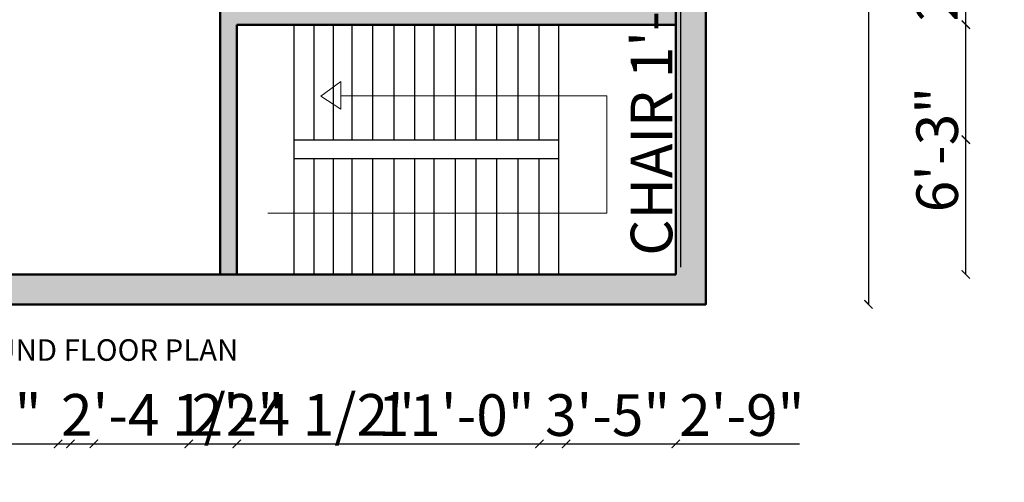
# Model space of a CAD drawing. Units: inches. Extents: x 2419 to 2878, y 1068 to 1713.
# Tile 8 of 20: x 2574 to 2870, y 1068 to 1207. Entities that reach past the tile are written whole.
import ezdxf

# ---------------------------------------------------------------- set-up
doc = ezdxf.new("R2010")
doc.units = ezdxf.units.IN
for name, color, linetype, lineweight in [('A-ANNO-DIMS', 2, 'Continuous', 18), ('A-ANNO-SYMB', 3, 'Continuous', 18), ('A-ANNO-TEXT', 7, 'Continuous', 25), ('A-FLOR-PRKG-PATT', 1, 'Continuous', 13), ('A-FLOR-STRS', 7, 'Continuous', 25), ('A-WALL', 7, 'Continuous', 50)]:
    doc.layers.add(name, color=color, linetype=linetype, lineweight=lineweight)
doc.layers.add('A-WALL-PATT', color=18, linetype='Continuous', lineweight=13, true_color=0x000000)
doc.styles.get("Standard").update_dxf_attribs({"font": 'arial.ttf'})
doc.dimstyles.new('ISO-25', dxfattribs={"dimtxt": 12.5, "dimasz": 2.5, "dimexe": 1.25, "dimexo": 0.625, "dimtad": 1, "dimdec": 0, "dimlunit": 4, "dimtxsty": 'Standard', "dimblk": 'ARCHTICK', "dimcen": 2.5, "dimse1": 1, "dimse2": 1, "dimclrd": 4, "dimadec": 0, "dimazin": 0, "dimtfac": 1, "dimtdec": 0, "dimtmove": 0, "dimatfit": 3, "dimfxl": 1, "dimarcsym": 0})

# ---------------------------------------------------------------- blocks, each defined once
blk = doc.blocks.new('_ArchTick')
at = {"color": 0, "linetype": 'ByBlock', "const_width": 0.15}
blk.add_lwpolyline([(-0.5, -0.5), (0.5, 0.5)], dxfattribs=at)
blk = doc.blocks.new('*D17')
at = {"layer": 'A-ANNO-DIMS', "color": 0, "lineweight": -2, "transparency": 16777216}
blk.add_line((2829.44, 1577.81), (2829.44, 1121.81), dxfattribs=at)
at = {"layer": 'Defpoints', "color": 0, "transparency": 16777216}
for p in [(2780.51, 1577.81), (2780.51, 1121.81), (2829.44, 1121.81)]:
    blk.add_point(p, dxfattribs=at)
at = {"layer": 'A-ANNO-DIMS', "color": 0, "lineweight": -2, "transparency": 16777216, "xscale": 2.5, "yscale": 2.5, "zscale": 2.5}
for p, rotation in [((2829.44, 1577.81), 90), ((2829.44, 1121.81), 270)]:
    blk.add_blockref('_ArchTick', p, dxfattribs=dict(at, rotation=rotation))
at = {"layer": 'A-ANNO-DIMS', "color": 0, "transparency": 16777216, "insert": (2822.42, 1349.81), "char_height": 12.5, "attachment_point": 5, "rotation": 90}
blk.add_mtext("38'", dxfattribs=at)
blk = doc.blocks.new('*D18')
at = {"layer": 'A-ANNO-DIMS', "color": 4, "lineweight": -2, "transparency": 16777216}
for p, q in [((2772.91, 1292.99), (2772.91, 1271.99)), ((2772.91, 1271.99), (2772.91, 1133))]:
    blk.add_line(p, q, dxfattribs=at)
at = {"layer": 'Defpoints', "color": 0, "transparency": 16777216}
for p in [(2769.76, 1292.99), (2769.76, 1271.99), (2772.91, 1271.99)]:
    blk.add_point(p, dxfattribs=at)
at = {"layer": 'A-ANNO-DIMS', "color": 4, "lineweight": -2, "transparency": 16777216, "xscale": 2.5, "yscale": 2.5, "zscale": 2.5}
for p, rotation in [((2772.91, 1292.99), 90), ((2772.91, 1271.99), 270)]:
    blk.add_blockref('_ArchTick', p, dxfattribs=dict(at, rotation=rotation))
at = {"layer": 'A-ANNO-DIMS', "color": 0, "transparency": 16777216, "insert": (2765.82, 1201.24), "char_height": 12.5, "attachment_point": 5, "rotation": 90}
blk.add_mtext('CHAIR 1\'-9" TYP.', dxfattribs=at)
blk = doc.blocks.new('*D34')
at = {"layer": 'A-ANNO-DIMS', "color": 4, "lineweight": -2, "transparency": 16777216}
blk.add_line((2639.51, 1079.92), (2771.51, 1079.92), dxfattribs=at)
at = {"layer": 'Defpoints', "color": 0, "transparency": 16777216}
for p in [(2639.51, 1130.81), (2771.51, 1130.81), (2771.51, 1079.92)]:
    blk.add_point(p, dxfattribs=at)
at = {"layer": 'A-ANNO-DIMS', "color": 4, "lineweight": -2, "transparency": 16777216, "xscale": 2.5, "yscale": 2.5, "zscale": 2.5, "rotation": 180}
blk.add_blockref('_ArchTick', (2639.51, 1079.92), dxfattribs=at)
at = {"layer": 'A-ANNO-DIMS', "color": 4, "lineweight": -2, "transparency": 16777216, "xscale": 2.5, "yscale": 2.5, "zscale": 2.5}
blk.add_blockref('_ArchTick', (2771.51, 1079.92), dxfattribs=at)
at = {"layer": 'A-ANNO-DIMS', "color": 0, "transparency": 16777216, "insert": (2705.51, 1086.93), "char_height": 12.5, "attachment_point": 5}
blk.add_mtext('11\'-0"', dxfattribs=at)
blk = doc.blocks.new('*D35')
at = {"layer": 'A-ANNO-DIMS', "color": 4, "lineweight": -2, "transparency": 16777216}
blk.add_line((2858.71, 1130.81), (2858.71, 1205.81), dxfattribs=at)
at = {"layer": 'Defpoints', "color": 0, "transparency": 16777216}
for p in [(2771.51, 1205.81), (2858.71, 1205.81), (2771.51, 1130.81)]:
    blk.add_point(p, dxfattribs=at)
at = {"layer": 'A-ANNO-DIMS', "color": 4, "lineweight": -2, "transparency": 16777216, "xscale": 2.5, "yscale": 2.5, "zscale": 2.5}
for p, rotation in [((2858.71, 1205.81), 90), ((2858.71, 1130.81), 270)]:
    blk.add_blockref('_ArchTick', p, dxfattribs=dict(at, rotation=rotation))
at = {"layer": 'A-ANNO-DIMS', "color": 0, "transparency": 16777216, "insert": (2851.7, 1168.31), "char_height": 12.5, "attachment_point": 5, "rotation": 90}
blk.add_mtext('6\'-3"', dxfattribs=at)
blk = doc.blocks.new('*D36')
at = {"layer": 'A-ANNO-DIMS', "color": 4, "lineweight": -2, "transparency": 16777216}
blk.add_line((2656.74, 1605.01), (2736.32, 1605.01), dxfattribs=at)
at = {"layer": 'Defpoints', "color": 0, "transparency": 16777216}
for p in [(2736.32, 1605.01), (2656.74, 1205.81), (2736.32, 1205.81)]:
    blk.add_point(p, dxfattribs=at)
at = {"layer": 'A-ANNO-DIMS', "color": 4, "lineweight": -2, "transparency": 16777216, "xscale": 2.5, "yscale": 2.5, "zscale": 2.5, "rotation": 180}
blk.add_blockref('_ArchTick', (2656.74, 1605.01), dxfattribs=at)
at = {"layer": 'A-ANNO-DIMS', "color": 4, "lineweight": -2, "transparency": 16777216, "xscale": 2.5, "yscale": 2.5, "zscale": 2.5}
blk.add_blockref('_ArchTick', (2736.32, 1605.01), dxfattribs=at)
at = {"layer": 'A-ANNO-DIMS', "color": 0, "transparency": 16777216, "insert": (2696.53, 1612.1), "char_height": 12.5, "attachment_point": 5}
blk.add_mtext('6\'-7 1/2"', dxfattribs=at)
blk = doc.blocks.new('*D37')
at = {"layer": 'A-ANNO-DIMS', "color": 4, "lineweight": -2, "transparency": 16777216}
for p, q in [((2736.32, 1605.01), (2771.51, 1605.01)), ((2771.51, 1605.01), (2818.42, 1605.01))]:
    blk.add_line(p, q, dxfattribs=at)
at = {"layer": 'Defpoints', "color": 0, "transparency": 16777216}
for p in [(2771.51, 1605.01), (2736.32, 1205.81), (2771.51, 1205.81)]:
    blk.add_point(p, dxfattribs=at)
at = {"layer": 'A-ANNO-DIMS', "color": 4, "lineweight": -2, "transparency": 16777216, "xscale": 2.5, "yscale": 2.5, "zscale": 2.5, "rotation": 180}
blk.add_blockref('_ArchTick', (2736.32, 1605.01), dxfattribs=at)
at = {"layer": 'A-ANNO-DIMS', "color": 4, "lineweight": -2, "transparency": 16777216, "xscale": 2.5, "yscale": 2.5, "zscale": 2.5}
blk.add_blockref('_ArchTick', (2771.51, 1605.01), dxfattribs=at)
at = {"layer": 'A-ANNO-DIMS', "color": 0, "transparency": 16777216, "insert": (2796.22, 1611.91), "char_height": 12.5, "attachment_point": 5}
blk.add_mtext('2\'-11"', dxfattribs=at)
blk = doc.blocks.new('*D38')
at = {"layer": 'A-ANNO-DIMS', "color": 4, "lineweight": -2, "transparency": 16777216}
for p, q in [((2444.31, 1165.6), (2444.31, 1212.51)), ((2444.31, 1130.81), (2444.31, 1165.6))]:
    blk.add_line(p, q, dxfattribs=at)
at = {"layer": 'Defpoints', "color": 0, "transparency": 16777216}
for p in [(2444.31, 1165.6), (2656.74, 1165.6), (2656.74, 1130.81)]:
    blk.add_point(p, dxfattribs=at)
at = {"layer": 'A-ANNO-DIMS', "color": 4, "lineweight": -2, "transparency": 16777216, "xscale": 2.5, "yscale": 2.5, "zscale": 2.5}
for p, rotation in [((2444.31, 1165.6), 90), ((2444.31, 1130.81), 270)]:
    blk.add_blockref('_ArchTick', p, dxfattribs=dict(at, rotation=rotation))
at = {"layer": 'A-ANNO-DIMS', "color": 0, "transparency": 16777216, "insert": (2437.41, 1190.3), "char_height": 12.5, "attachment_point": 5, "rotation": 90}
blk.add_mtext('2\'-11"', dxfattribs=at)
blk = doc.blocks.new('*D39')
at = {"layer": 'A-ANNO-DIMS', "color": 4, "lineweight": -2, "transparency": 16777216}
for p, q in [((2662.74, 1605.01), (2668.59, 1605.01)), ((2668.59, 1605.01), (2705.56, 1605.01))]:
    blk.add_line(p, q, dxfattribs=at)
at = {"layer": 'Defpoints', "color": 0, "transparency": 16777216}
for p in [(2668.59, 1605.01), (2662.74, 1165.6), (2668.59, 1165.6)]:
    blk.add_point(p, dxfattribs=at)
at = {"layer": 'A-ANNO-DIMS', "color": 4, "lineweight": -2, "transparency": 16777216, "xscale": 2.5, "yscale": 2.5, "zscale": 2.5, "rotation": 180}
blk.add_blockref('_ArchTick', (2662.74, 1605.01), dxfattribs=at)
at = {"layer": 'A-ANNO-DIMS', "color": 4, "lineweight": -2, "transparency": 16777216, "xscale": 2.5, "yscale": 2.5, "zscale": 2.5}
blk.add_blockref('_ArchTick', (2668.59, 1605.01), dxfattribs=at)
at = {"layer": 'A-ANNO-DIMS', "color": 0, "transparency": 16777216, "insert": (2688.32, 1612.02), "char_height": 12.5, "attachment_point": 5}
blk.add_mtext('0\'-6"', dxfattribs=at)
blk = doc.blocks.new('*D40')
at = {"layer": 'A-ANNO-DIMS', "color": 4, "lineweight": -2, "transparency": 16777216}
for p, q in [((2858.71, 1205.81), (2858.71, 1281.84)), ((2858.71, 1171.28), (2858.71, 1205.81))]:
    blk.add_line(p, q, dxfattribs=at)
at = {"layer": 'Defpoints', "color": 0, "transparency": 16777216}
for p in [(2736.32, 1205.81), (2858.71, 1205.81), (2736.32, 1171.28)]:
    blk.add_point(p, dxfattribs=at)
at = {"layer": 'A-ANNO-DIMS', "color": 4, "lineweight": -2, "transparency": 16777216, "xscale": 2.5, "yscale": 2.5, "zscale": 2.5}
for p, rotation in [((2858.71, 1205.81), 90), ((2858.71, 1171.28), 270)]:
    blk.add_blockref('_ArchTick', p, dxfattribs=dict(at, rotation=rotation))
at = {"layer": 'A-ANNO-DIMS', "color": 0, "transparency": 16777216, "insert": (2851.63, 1245.08), "char_height": 12.5, "attachment_point": 5, "rotation": 90}
blk.add_mtext('2\'-10 1/2"', dxfattribs=at)
blk = doc.blocks.new('*D44')
at = {"layer": 'A-ANNO-DIMS', "color": 4, "lineweight": -2, "transparency": 16777216}
for p, q in [((2557.3, 1079.92), (2585.82, 1079.92)), ((2585.82, 1079.92), (2652.14, 1079.92))]:
    blk.add_line(p, q, dxfattribs=at)
at = {"layer": 'Defpoints', "color": 0, "transparency": 16777216}
for p in [(2557.3, 1408.81), (2585.82, 1408.81), (2585.82, 1079.92)]:
    blk.add_point(p, dxfattribs=at)
at = {"layer": 'A-ANNO-DIMS', "color": 4, "lineweight": -2, "transparency": 16777216, "xscale": 2.5, "yscale": 2.5, "zscale": 2.5, "rotation": 180}
blk.add_blockref('_ArchTick', (2557.3, 1079.92), dxfattribs=at)
at = {"layer": 'A-ANNO-DIMS', "color": 4, "lineweight": -2, "transparency": 16777216, "xscale": 2.5, "yscale": 2.5, "zscale": 2.5}
blk.add_blockref('_ArchTick', (2585.82, 1079.92), dxfattribs=at)
at = {"layer": 'A-ANNO-DIMS', "color": 0, "transparency": 16777216, "insert": (2620.23, 1087.01), "char_height": 12.5, "attachment_point": 5}
blk.add_mtext('2\'-4 1/2"', dxfattribs=at)
blk = doc.blocks.new('*D45')
at = {"layer": 'A-ANNO-DIMS', "color": 4, "lineweight": -2, "transparency": 16777216}
for p, q in [((2596.57, 1079.92), (2625.09, 1079.92)), ((2625.09, 1079.92), (2691.41, 1079.92))]:
    blk.add_line(p, q, dxfattribs=at)
at = {"layer": 'Defpoints', "color": 0, "transparency": 16777216}
for p in [(2596.57, 1408.81), (2625.09, 1408.81), (2625.09, 1079.92)]:
    blk.add_point(p, dxfattribs=at)
at = {"layer": 'A-ANNO-DIMS', "color": 4, "lineweight": -2, "transparency": 16777216, "xscale": 2.5, "yscale": 2.5, "zscale": 2.5, "rotation": 180}
blk.add_blockref('_ArchTick', (2596.57, 1079.92), dxfattribs=at)
at = {"layer": 'A-ANNO-DIMS', "color": 4, "lineweight": -2, "transparency": 16777216, "xscale": 2.5, "yscale": 2.5, "zscale": 2.5}
blk.add_blockref('_ArchTick', (2625.09, 1079.92), dxfattribs=at)
at = {"layer": 'A-ANNO-DIMS', "color": 0, "transparency": 16777216, "insert": (2659.5, 1087.01), "char_height": 12.5, "attachment_point": 5}
blk.add_mtext('2\'-4 1/2"', dxfattribs=at)
blk = doc.blocks.new('*D51')
at = {"layer": 'A-ANNO-DIMS', "color": 4, "lineweight": -2, "transparency": 16777216}
for p, q in [((2738.51, 1079.92), (2771.51, 1079.92)), ((2771.51, 1079.92), (2808.71, 1079.92))]:
    blk.add_line(p, q, dxfattribs=at)
at = {"layer": 'Defpoints', "color": 0, "transparency": 16777216}
for p in [(2738.51, 1447.89), (2771.51, 1437.39), (2771.51, 1079.92)]:
    blk.add_point(p, dxfattribs=at)
at = {"layer": 'A-ANNO-DIMS', "color": 4, "lineweight": -2, "transparency": 16777216, "xscale": 2.5, "yscale": 2.5, "zscale": 2.5, "rotation": 180}
blk.add_blockref('_ArchTick', (2738.51, 1079.92), dxfattribs=at)
at = {"layer": 'A-ANNO-DIMS', "color": 4, "lineweight": -2, "transparency": 16777216, "xscale": 2.5, "yscale": 2.5, "zscale": 2.5}
blk.add_blockref('_ArchTick', (2771.51, 1079.92), dxfattribs=at)
at = {"layer": 'A-ANNO-DIMS', "color": 0, "transparency": 16777216, "insert": (2791.36, 1086.93), "char_height": 12.5, "attachment_point": 5}
blk.add_mtext('2\'-9"', dxfattribs=at)
blk = doc.blocks.new('*D56')
at = {"layer": 'A-ANNO-DIMS', "color": 4, "lineweight": -2, "transparency": 16777216}
for p, q in [((2480.51, 1079.92), (2503.97, 1079.92)), ((2503.97, 1079.92), (2578.61, 1079.92))]:
    blk.add_line(p, q, dxfattribs=at)
at = {"layer": 'Defpoints', "color": 0, "transparency": 16777216}
for p in [(2480.51, 1507.81), (2503.97, 1494.85), (2503.97, 1079.92)]:
    blk.add_point(p, dxfattribs=at)
at = {"layer": 'A-ANNO-DIMS', "color": 4, "lineweight": -2, "transparency": 16777216, "xscale": 2.5, "yscale": 2.5, "zscale": 2.5, "rotation": 180}
blk.add_blockref('_ArchTick', (2480.51, 1079.92), dxfattribs=at)
at = {"layer": 'A-ANNO-DIMS', "color": 4, "lineweight": -2, "transparency": 16777216, "xscale": 2.5, "yscale": 2.5, "zscale": 2.5}
blk.add_blockref('_ArchTick', (2503.97, 1079.92), dxfattribs=at)
at = {"layer": 'A-ANNO-DIMS', "color": 0, "transparency": 16777216, "insert": (2542.54, 1087.01), "char_height": 12.5, "attachment_point": 5}
blk.add_mtext('1\'-11 1/2"', dxfattribs=at)
blk = doc.blocks.new('*D59')
at = {"layer": 'A-ANNO-DIMS', "color": 4, "lineweight": -2, "transparency": 16777216}
blk.add_line((2480.51, 1079.92), (2589.51, 1079.92), dxfattribs=at)
at = {"layer": 'Defpoints', "color": 0, "transparency": 16777216}
for p in [(2480.51, 1414.81), (2589.51, 1414.81), (2589.51, 1079.92)]:
    blk.add_point(p, dxfattribs=at)
at = {"layer": 'A-ANNO-DIMS', "color": 4, "lineweight": -2, "transparency": 16777216, "xscale": 2.5, "yscale": 2.5, "zscale": 2.5, "rotation": 180}
blk.add_blockref('_ArchTick', (2480.51, 1079.92), dxfattribs=at)
at = {"layer": 'A-ANNO-DIMS', "color": 4, "lineweight": -2, "transparency": 16777216, "xscale": 2.5, "yscale": 2.5, "zscale": 2.5}
blk.add_blockref('_ArchTick', (2589.51, 1079.92), dxfattribs=at)
at = {"layer": 'A-ANNO-DIMS', "color": 0, "transparency": 16777216, "insert": (2535.01, 1086.93), "char_height": 12.5, "attachment_point": 5}
blk.add_mtext('9\'-1"', dxfattribs=at)
blk = doc.blocks.new('*D61')
at = {"layer": 'A-ANNO-DIMS', "color": 4, "lineweight": -2, "transparency": 16777216}
blk.add_line((2730.51, 1079.92), (2771.51, 1079.92), dxfattribs=at)
at = {"layer": 'Defpoints', "color": 0, "transparency": 16777216}
for p in [(2730.51, 1414.81), (2771.51, 1414.81), (2771.51, 1079.92)]:
    blk.add_point(p, dxfattribs=at)
at = {"layer": 'A-ANNO-DIMS', "color": 4, "lineweight": -2, "transparency": 16777216, "xscale": 2.5, "yscale": 2.5, "zscale": 2.5, "rotation": 180}
blk.add_blockref('_ArchTick', (2730.51, 1079.92), dxfattribs=at)
at = {"layer": 'A-ANNO-DIMS', "color": 4, "lineweight": -2, "transparency": 16777216, "xscale": 2.5, "yscale": 2.5, "zscale": 2.5}
blk.add_blockref('_ArchTick', (2771.51, 1079.92), dxfattribs=at)
at = {"layer": 'A-ANNO-DIMS', "color": 0, "transparency": 16777216, "insert": (2751.01, 1086.94), "char_height": 12.5, "attachment_point": 5}
blk.add_mtext('3\'-5"', dxfattribs=at)

msp = doc.modelspace()

# ---------------------------------------------------------------- hatches: boundary and pattern name
at = {"layer": 'A-FLOR-PRKG-PATT'}
h = msp.add_hatch(color=256, dxfattribs=at)
h.dxf.hatch_style = 1
edge = h.paths.add_edge_path()
edge.add_ellipse((2561.37, 1279.45), major_axis=(3.99, 0), ratio=0.842304, start_angle=0.6466, end_angle=90)
edge.add_line((2561.37, 1282.81), (2511.57, 1282.81))
edge.add_ellipse((2511.57, 1279.45), major_axis=(3.99, 0), ratio=0.842304, start_angle=90, end_angle=179.3534)
edge.add_ellipse((10560.89, 1188.62), major_axis=(-8054.03, 0), ratio=0.8423039, start_angle=-0.646554, end_angle=-0.628237)
edge.add_ellipse((2509.23, 1276.91), major_axis=(1.69, 0), ratio=0.842304, start_angle=179.3718, end_angle=248.4648)
edge.add_ellipse((10560.33, 1188.62), major_axis=(8052.29, 0), ratio=0.8423039, start_angle=179.353446, end_angle=179.381357, ccw=False)
edge.add_ellipse((2511.01, 1279.45), major_axis=(2.25, 0), ratio=0.842304, start_angle=90, end_angle=179.3534, ccw=False)
edge.add_line((2511.01, 1281.35), (2561.94, 1281.35))
edge.add_ellipse((2561.94, 1279.45), major_axis=(-2.25, 0), ratio=0.842304, start_angle=180.6466, end_angle=270, ccw=False)
edge.add_ellipse((-5487.38, 1188.62), major_axis=(8052.29, 0), ratio=0.8423039, start_angle=0.528271, end_angle=0.646554, ccw=False)
edge.add_ellipse((2563.71, 1276.91), major_axis=(-1.69, 0), ratio=0.842304, start_angle=111.5352, end_angle=180.6282)
edge.add_ellipse((-5487.95, 1188.62), major_axis=(-8054.03, 0), ratio=0.8423039, start_angle=180.628237, end_angle=180.646554)
edge = h.paths.add_edge_path()
edge.add_ellipse((2564.91, 1261.91), major_axis=(-1.12, 0), ratio=0.842304, start_angle=180, end_angle=270)
edge.add_line((2564.91, 1262.86), (2564.43, 1262.86))
edge.add_ellipse((-5487.38, 1188.62), major_axis=(8052.29, 0), ratio=0.8423039, start_angle=0.383867, end_angle=0.528271, ccw=False)
edge.add_line((2564.65, 1242.56), (2564.91, 1242.56))
edge.add_ellipse((2564.91, 1243.51), major_axis=(-1.12, 0), ratio=0.842304, start_angle=90, end_angle=180)
edge.add_line((2566.03, 1243.51), (2566.03, 1261.91))
edge = h.paths.add_edge_path()
edge.add_ellipse((2564.91, 1174.99), major_axis=(1.12, 0), ratio=0.842304, start_angle=0, end_angle=90)
edge.add_line((2564.91, 1175.94), (2564.89, 1175.94))
edge.add_ellipse((-5487.38, 1188.62), major_axis=(8052.29, 0), ratio=0.8423039, start_angle=-0.134987, end_angle=-0.090229, ccw=False)
edge.add_ellipse((2163.34, 1170.91), major_axis=(401.54, 0), ratio=0.842304, start_angle=-2.18, end_angle=-0.1356, ccw=False)
edge.add_line((2564.47, 1155.64), (2564.91, 1155.64))
edge.add_ellipse((2564.91, 1156.59), major_axis=(-1.12, 0), ratio=0.842304, start_angle=90, end_angle=180)
edge.add_line((2566.03, 1156.59), (2566.03, 1174.99))
h.paths.add_polyline_path([(2574.48, 1207.45), (2633.94, 1207.45), (2633.94, 1217.37), (2574.48, 1217.37)], flags=9)
h.paths.add_polyline_path([(2574.45, 1217.83), (2610.47, 1217.83), (2610.47, 1227.88), (2574.45, 1227.88)], flags=9)
h.paths.add_polyline_path([(2672.43, 1304.02), (2718.62, 1304.02), (2718.62, 1313.94), (2672.43, 1313.94)], flags=9)
h.paths.add_polyline_path([(2672.4, 1314.4), (2750.13, 1314.4), (2750.13, 1324.45), (2672.4, 1324.45)], flags=9)
h.paths.add_polyline_path([(2500.43, 1374.44), (2544.8, 1374.44), (2544.8, 1384.36), (2500.43, 1384.36)], flags=9)
h.paths.add_polyline_path([(2500.41, 1384.82), (2566.08, 1384.82), (2566.08, 1394.87), (2500.41, 1394.87)], flags=9)
h.paths.add_polyline_path([(2738.93, 1376.75), (2778.27, 1376.75), (2778.27, 1386.67), (2738.93, 1386.67)], flags=9)
h.paths.add_polyline_path([(2659.12, 1357.8), (2703.49, 1357.8), (2703.49, 1367.72), (2659.12, 1367.72)], flags=9)
h.paths.add_polyline_path([(2659.1, 1368.18), (2694.11, 1368.18), (2694.11, 1378.23), (2659.1, 1378.23)], flags=9)
h.paths.add_polyline_path([(2730.12, 1466.07), (2769.46, 1466.07), (2769.46, 1475.99), (2730.12, 1475.99)], flags=9)
h.paths.add_polyline_path([(2730.1, 1476.45), (2765.12, 1476.45), (2765.12, 1486.5), (2730.1, 1486.5)], flags=9)
h.paths.add_polyline_path([(2730.38, 1518.65), (2761.48, 1518.65), (2761.48, 1528.57), (2730.38, 1528.57)], flags=9)
h.paths.add_polyline_path([(2730.36, 1529.03), (2780.96, 1529.03), (2780.96, 1539.07), (2730.36, 1539.07)], flags=9)
h.paths.add_polyline_path([(2629.32, 1455.19), (2688.78, 1455.19), (2688.78, 1465.11), (2629.32, 1465.11)], flags=9)
h.paths.add_polyline_path([(2629.3, 1465.57), (2681.9, 1465.57), (2681.9, 1475.62), (2629.3, 1475.62)], flags=9)
h.paths.add_polyline_path([(2513.23, 1456.48), (2562.63, 1456.48), (2562.63, 1466.4), (2513.23, 1466.4)], flags=9)
h.paths.add_polyline_path([(2513.21, 1466.86), (2556.26, 1466.86), (2556.26, 1476.91), (2513.21, 1476.91)], flags=9)
h.paths.add_polyline_path([(2488.87, 1521.54), (2519.97, 1521.54), (2519.97, 1531.46), (2488.87, 1531.46)], flags=9)
h.paths.add_polyline_path([(2536.55, 1543.51), (2580.92, 1543.51), (2580.92, 1553.43), (2536.55, 1553.43)], flags=9)
h.paths.add_polyline_path([(2536.56, 1553.92), (2573.53, 1553.92), (2573.53, 1563.8), (2536.56, 1563.8)], flags=9)
at = {"layer": 'A-WALL-PATT'}
h = msp.add_hatch(color=256, dxfattribs=at)
h.dxf.hatch_style = 1
h.paths.add_polyline_path([(2780.51, 1577.81), (2471.51, 1577.81), (2471.51, 1121.81), (2780.51, 1121.81)])
h.paths.add_polyline_path([(2480.51, 1568.81), (2771.51, 1568.81), (2771.51, 1130.81), (2480.51, 1130.81)], flags=16)
h.paths.add_polyline_path([(2528.51, 1568.81), (2528.51, 1512.81), (2594.51, 1512.81), (2594.51, 1414.81), (2596.57, 1414.81), (2596.57, 1441.61), (2597.82, 1441.61), (2597.82, 1441.58, -0.384016), (2625.03, 1414.81), (2725.51, 1414.81), (2725.51, 1567.55), (2728.3, 1567.55), (2746.89, 1567.55), (2746.89, 1566.73), (2746.87, 1566.73, -0.367216), (2730.51, 1549.09), (2730.51, 1512.81), (2750.85, 1512.81), (2750.85, 1510.03, -0.401453), (2733.08, 1491.46), (2733.08, 1491.44), (2732.27, 1491.44), (2732.27, 1507.81), (2730.51, 1507.81), (2730.51, 1408.81), (2736.51, 1408.81), (2736.51, 1349.81), (2632.51, 1349.81), (2632.51, 1408.81), (2528.51, 1408.81), (2528.51, 1414.81), (2503.97, 1414.81), (2503.97, 1494.85), (2558.38, 1494.85), (2558.38, 1507.81), (2529.96, 1507.81, -0.414214), (2530.82, 1506.96), (2530.82, 1497.26, -0.414214), (2529.96, 1496.4), (2514.56, 1496.4, -0.414214), (2513.7, 1497.26), (2513.7, 1506.96, -0.414214), (2514.56, 1507.81), (2528.51, 1507.81), (2528.51, 1512.81), (2480.51, 1512.81)], flags=0)
h.paths.add_polyline_path([(2516.26, 1507.81), (2528.26, 1507.81), (2528.26, 1505.81), (2523.42, 1505.81), (2524.07, 1504.67), (2529.39, 1504.67, -0.414214), (2529.96, 1504.1), (2529.96, 1497.83, -0.414214), (2529.39, 1497.26), (2515.13, 1497.26, -0.414214), (2514.56, 1497.83), (2514.56, 1504.1, -0.414214), (2515.13, 1504.67), (2520.69, 1504.67), (2521.34, 1505.81), (2516.26, 1505.81)], flags=0)
h.paths.add_polyline_path([(2522.02, 1505.53), (2522.82, 1507.32, -0.65506), (2522.25, 1506.06), (2522.19, 1505.93), (2522.43, 1505.53)], flags=0)
h.paths.add_polyline_path([(2522.83, 1500.97, -1), (2521.69, 1500.97, -1)], flags=0)
h.paths.add_polyline_path([(2522.55, 1500.97, -1), (2521.98, 1500.97, -1)], flags=0)
h.paths.add_polyline_path([(2482.01, 1470.63), (2499.89, 1470.63), (2499.89, 1448.27), (2482.01, 1448.27), (2482.01, 1452.74), (2481.26, 1452.74), (2481.26, 1449.76), (2480.51, 1449.76), (2480.51, 1469.14), (2481.26, 1469.14), (2481.26, 1466.16), (2482.01, 1466.16)], flags=0)
h.paths.add_polyline_path([(2488.71, 1466.16, -1), (2484.24, 1466.16, -1)], flags=0)
h.paths.add_polyline_path([(2496.17, 1466.16, -1), (2490.2, 1466.16, -1)], flags=0)
h.paths.add_polyline_path([(2487.97, 1466.16, -1), (2484.99, 1466.16, -1)], flags=0)
h.paths.add_polyline_path([(2495.42, 1466.16, -1), (2490.95, 1466.16, -1)], flags=0)
h.paths.add_polyline_path([(2487.22, 1466.16, -1), (2485.73, 1466.16, -1)], flags=0)
h.paths.add_polyline_path([(2494.68, 1466.16, -1), (2491.69, 1466.16, -1)], flags=0)
h.paths.add_polyline_path([(2499.11, 1468, -1), (2497.98, 1468, -1)], flags=0)
h.paths.add_polyline_path([(2493.93, 1466.16, -1), (2492.44, 1466.16, -1)], flags=0)
h.paths.add_polyline_path([(2499.37, 1463.71, -1), (2498.17, 1463.71, -1)], flags=0)
h.paths.add_polyline_path([(2484.24, 1461.69), (2496.17, 1461.69), (2496.17, 1457.22), (2484.24, 1457.22)], flags=0)
h.paths.add_polyline_path([(2484.99, 1460.94), (2495.42, 1460.94), (2495.42, 1457.96), (2484.99, 1457.96)], flags=0)
h.paths.add_polyline_path([(2586.88, 1510.03), (2587.69, 1510.03), (2587.69, 1491.44), (2586.88, 1491.44)], flags=0)
h.paths.add_polyline_path([(2499.26, 1459.41, -1), (2498.2, 1459.41, -1)], flags=0)
h.paths.add_polyline_path([(2489.46, 1452.74, -1), (2483.5, 1452.74, -1)], flags=0)
h.paths.add_polyline_path([(2557.3, 1408.81), (2557.3, 1413.09, -0.401453), (2584.57, 1441.58), (2584.57, 1441.61), (2585.82, 1441.61), (2585.82, 1413.09), (2585.82, 1408.81)], flags=0)
h.paths.add_polyline_path([(2488.71, 1452.74, -1), (2484.24, 1452.74, -1)], flags=0)
h.paths.add_polyline_path([(2495.42, 1452.74, -1), (2490.95, 1452.74, -1)], flags=0)
h.paths.add_polyline_path([(2487.97, 1452.74, -1), (2484.99, 1452.74, -1)], flags=0)
h.paths.add_polyline_path([(2494.68, 1452.74, -1), (2491.69, 1452.74, -1)], flags=0)
h.paths.add_polyline_path([(2487.22, 1452.74, -1), (2485.73, 1452.74, -1)], flags=0)
h.paths.add_polyline_path([(2499.18, 1454.44, -1), (2497.9, 1454.44, -1)], flags=0)
h.paths.add_polyline_path([(2493.93, 1452.74, -1), (2492.44, 1452.74, -1)], flags=0)
h.paths.add_polyline_path([(2499.3, 1450.64, -1), (2497.79, 1450.64, -1)], flags=0)
h.paths.add_polyline_path([(2619.13, 1558.89, -1), (2605.13, 1558.89, -1)], flags=0)
h.paths.add_polyline_path([(2609.13, 1558.89), (2612.13, 1561.89), (2615.13, 1558.89), (2612.13, 1555.89)], flags=0)
h.paths.add_polyline_path([(2611.13, 1558.89, -1), (2613.13, 1558.89, -1)], flags=0)
h.paths.add_polyline_path([(2633.68, 1568.81), (2693.68, 1568.81), (2693.68, 1488.81), (2633.68, 1488.81)], flags=0)
h.paths.add_polyline_path([(2641.68, 1554.41), (2641.68, 1567.61), (2662.48, 1567.61), (2662.48, 1554.41), (2664.88, 1554.41), (2664.88, 1567.61), (2685.68, 1567.61), (2685.68, 1552.41), (2680.48, 1552.41), (2693.68, 1539.21), (2678.48, 1539.21), (2678.48, 1554.41)], flags=0)
h.paths.add_polyline_path([(2637.51, 1408.81), (2731.51, 1408.81), (2731.51, 1354.81), (2637.51, 1354.81), (2637.51, 1357.98), (2635.3, 1357.98), (2635.3, 1358.79), (2637.51, 1358.79)], flags=0)
h.paths.add_polyline_path([(2717.17, 1559.64, -1), (2703.17, 1559.64, -1)], flags=0)
h.paths.add_polyline_path([(2707.17, 1559.64), (2710.17, 1562.64), (2713.17, 1559.64), (2710.17, 1556.64)], flags=0)
h.paths.add_polyline_path([(2709.17, 1559.64, -1), (2711.17, 1559.64, -1)], flags=0)
h.paths.add_polyline_path([(2685.38, 1408.81), (2706.38, 1408.81), (2706.38, 1400.81), (2699.88, 1400.81), (2701.88, 1394.81, -0.501323), (2696.92, 1375.95, -0.132891), (2694.83, 1375.95, -0.501317), (2689.88, 1394.81), (2691.88, 1400.81), (2688.88, 1400.81), (2688.88, 1399.31), (2685.88, 1399.31), (2685.88, 1400.31), (2687.88, 1400.31), (2687.88, 1400.81), (2685.38, 1400.81)], flags=0)
h.paths.add_polyline_path([(2687.38, 1407.81), (2704.38, 1407.81, -0.5), (2705.38, 1406.81), (2705.38, 1402.81, -0.5), (2704.38, 1401.81), (2687.38, 1401.81, -0.5), (2686.38, 1402.81), (2686.38, 1406.81, -0.5)], flags=0)
h.paths.add_polyline_path([(2639.51, 1205.81), (2634.51, 1205.81), (2634.51, 1293.81), (2637.51, 1293.81), (2639.51, 1293.81)], flags=0)
h.paths.add_polyline_path([(2691.88, 1394.81), (2699.88, 1394.81, -0.48008), (2697.52, 1377.29, -0.215004), (2694.23, 1377.29, -0.48008)], flags=0)
h.paths.add_polyline_path([(2757.51, 1453.89), (2763.51, 1451.89), (2763.51, 1454.89), (2762.01, 1454.89), (2762.01, 1457.89), (2763.01, 1457.89), (2763.01, 1455.89), (2763.51, 1455.89), (2763.51, 1458.39), (2771.51, 1458.39), (2771.51, 1437.39), (2763.51, 1437.39), (2763.51, 1443.89), (2757.51, 1441.89, -0.501323), (2738.65, 1446.85, -0.132891), (2738.65, 1448.94, -0.501317)], flags=0)
h.paths.add_polyline_path([(2739.99, 1449.54, -0.48008), (2757.51, 1451.89), (2757.51, 1443.89, -0.48008), (2739.99, 1446.25, -0.215004)], flags=0)
h.paths.add_polyline_path([(2765.51, 1457.39), (2769.51, 1457.39, -0.5), (2770.51, 1456.39), (2770.51, 1439.39, -0.5), (2769.51, 1438.39), (2765.51, 1438.39, -0.5), (2764.51, 1439.39), (2764.51, 1456.39, -0.5)], flags=0)
h = msp.add_hatch(color=256, dxfattribs=at)
h.dxf.hatch_style = 1
h.paths.add_polyline_path([(2771.51, 1354.81), (2736.51, 1354.81), (2736.51, 1408.81), (2771.51, 1408.81), (2771.51, 1414.81), (2625.03, 1414.81, -0.015108), (2625.09, 1413.09), (2625.09, 1408.81), (2632.51, 1408.81), (2632.51, 1376.56), (2635.3, 1376.56, -0.029838), (2637.51, 1376.43), (2637.51, 1408.81), (2731.51, 1408.81), (2731.51, 1354.81), (2637.51, 1354.81), (2637.51, 1357.98), (2635.3, 1357.98), (2632.51, 1357.98), (2632.51, 1349.81), (2771.51, 1349.81)])
h.paths.add_polyline_path([(2639.51, 1298.81), (2637.51, 1298.81), (2480.51, 1298.81), (2480.51, 1293.81), (2637.51, 1293.81), (2639.51, 1293.81)])
h.paths.add_polyline_path([(2639.51, 1293.81), (2637.51, 1293.81), (2634.51, 1293.81), (2634.51, 1244.65), (2638.79, 1244.65, -0.006332), (2639.51, 1244.64)])
h.paths.add_polyline_path([(2639.51, 1205.81), (2771.51, 1205.81), (2771.51, 1210.81), (2639.51, 1210.81), (2639.51, 1216.13), (2638.79, 1216.13), (2634.51, 1216.13), (2634.51, 1130.81), (2639.51, 1130.81)])
h.paths.add_polyline_path([(2596.57, 1413.09), (2596.57, 1414.81), (2585.82, 1414.81), (2585.82, 1413.09), (2585.82, 1408.81), (2596.57, 1408.81)])
h.paths.add_polyline_path([(2557.3, 1413.09, -0.015108), (2557.35, 1414.81), (2480.51, 1414.81), (2480.51, 1408.81), (2557.3, 1408.81)])
h.paths.add_polyline_path([(2574.48, 1207.45), (2633.94, 1207.45), (2633.94, 1217.37), (2574.48, 1217.37)], flags=9)
h.paths.add_polyline_path([(2574.45, 1217.83), (2610.47, 1217.83), (2610.47, 1227.88), (2574.45, 1227.88)], flags=9)
h.paths.add_polyline_path([(2672.43, 1304.02), (2718.62, 1304.02), (2718.62, 1313.94), (2672.43, 1313.94)], flags=9)
h.paths.add_polyline_path([(2672.4, 1314.4), (2750.13, 1314.4), (2750.13, 1324.45), (2672.4, 1324.45)], flags=9)
h.paths.add_polyline_path([(2500.43, 1374.44), (2544.8, 1374.44), (2544.8, 1384.36), (2500.43, 1384.36)], flags=9)
h.paths.add_polyline_path([(2500.41, 1384.82), (2566.08, 1384.82), (2566.08, 1394.87), (2500.41, 1394.87)], flags=9)
h.paths.add_polyline_path([(2738.93, 1376.75), (2778.27, 1376.75), (2778.27, 1386.67), (2738.93, 1386.67)], flags=9)
h.paths.add_polyline_path([(2659.12, 1357.8), (2703.49, 1357.8), (2703.49, 1367.72), (2659.12, 1367.72)], flags=25)
h.paths.add_polyline_path([(2659.1, 1368.18), (2694.11, 1368.18), (2694.11, 1378.23), (2659.1, 1378.23)], flags=25)
h.paths.add_polyline_path([(2730.12, 1466.07), (2769.46, 1466.07), (2769.46, 1475.99), (2730.12, 1475.99)], flags=9)
h.paths.add_polyline_path([(2730.1, 1476.45), (2765.12, 1476.45), (2765.12, 1486.5), (2730.1, 1486.5)], flags=9)
h.paths.add_polyline_path([(2730.38, 1518.65), (2761.48, 1518.65), (2761.48, 1528.57), (2730.38, 1528.57)], flags=9)
h.paths.add_polyline_path([(2730.36, 1529.03), (2780.96, 1529.03), (2780.96, 1539.07), (2730.36, 1539.07)], flags=9)
h.paths.add_polyline_path([(2629.32, 1455.19), (2688.78, 1455.19), (2688.78, 1465.11), (2629.32, 1465.11)], flags=9)
h.paths.add_polyline_path([(2629.3, 1465.57), (2681.9, 1465.57), (2681.9, 1475.62), (2629.3, 1475.62)], flags=9)
h.paths.add_polyline_path([(2513.23, 1456.48), (2562.63, 1456.48), (2562.63, 1466.4), (2513.23, 1466.4)], flags=9)
h.paths.add_polyline_path([(2513.21, 1466.86), (2556.26, 1466.86), (2556.26, 1476.91), (2513.21, 1476.91)], flags=9)
h.paths.add_polyline_path([(2488.87, 1521.54), (2519.97, 1521.54), (2519.97, 1531.46), (2488.87, 1531.46)], flags=9)
h.paths.add_polyline_path([(2536.55, 1543.51), (2580.92, 1543.51), (2580.92, 1553.43), (2536.55, 1553.43)], flags=9)
h.paths.add_polyline_path([(2536.56, 1553.92), (2573.53, 1553.92), (2573.53, 1563.8), (2536.56, 1563.8)], flags=9)

# ---------------------------------------------------------------- linework, layer by layer
at = {"layer": 'A-ANNO-SYMB'}
for p, q in [((2670.85, 1188.73), (2664.84, 1184.37)), ((2670.85, 1184.48), (2670.85, 1188.73)), ((2664.84, 1184.37), (2670.85, 1180.48)), ((2750.76, 1184.48), (2670.85, 1184.48)), ((2670.85, 1180.48), (2670.85, 1184.48)), ((2750.76, 1149.19), (2750.76, 1184.48)), ((2648.83, 1149.19), (2750.76, 1149.19))]:
    msp.add_line(p, q, dxfattribs=at)
at = {"layer": 'A-FLOR-STRS'}
for p, q in [((2656.74, 1130.81), (2656.74, 1205.81)), ((2662.74, 1171.28), (2662.74, 1205.81)), ((2668.59, 1171.28), (2668.59, 1205.81)), ((2674.26, 1171.28), (2674.26, 1205.81)), ((2680.47, 1171.28), (2680.47, 1205.81)), ((2686.85, 1171.28), (2686.85, 1205.81)), ((2693.06, 1171.28), (2693.06, 1205.81)), ((2698.91, 1171.28), (2698.91, 1205.81)), ((2705.29, 1171.28), (2705.29, 1205.81)), ((2711.5, 1171.28), (2711.5, 1205.81)), ((2717.7, 1171.28), (2717.7, 1205.81)), ((2724.09, 1171.28), (2724.09, 1205.81)), ((2730.47, 1171.28), (2730.47, 1205.81)), ((2736.32, 1130.81), (2736.32, 1205.81)), ((2656.74, 1171.28), (2736.32, 1171.28)), ((2656.74, 1165.6), (2736.32, 1165.6)), ((2662.74, 1130.81), (2662.74, 1165.6)), ((2668.59, 1130.81), (2668.59, 1165.6)), ((2674.26, 1130.81), (2674.26, 1165.6)), ((2680.47, 1130.81), (2680.47, 1165.6)), ((2686.85, 1130.81), (2686.85, 1165.6)), ((2693.06, 1130.81), (2693.06, 1165.6)), ((2698.91, 1130.81), (2698.91, 1165.6)), ((2705.29, 1130.81), (2705.29, 1165.6)), ((2711.5, 1130.81), (2711.5, 1165.6)), ((2717.7, 1130.81), (2717.7, 1165.6)), ((2724.09, 1130.81), (2724.09, 1165.6)), ((2730.47, 1130.81), (2730.47, 1165.6))]:
    msp.add_line(p, q, dxfattribs=at)
at = {"layer": 'A-WALL'}
for p, q in [((2771.51, 1568.81), (2771.51, 1130.81)), ((2634.51, 1216.13), (2634.51, 1130.81)), ((2639.51, 1205.81), (2771.51, 1205.81)), ((2639.51, 1205.81), (2639.51, 1130.81)), ((2771.51, 1130.81), (2480.51, 1130.81))]:
    msp.add_line(p, q, dxfattribs=at)
msp.add_lwpolyline([(2471.51, 1577.81), (2780.51, 1577.81), (2780.51, 1121.81), (2471.51, 1121.81)], close=True, dxfattribs=at)

# ---------------------------------------------------------------- texts
at = {"layer": 'A-ANNO-TEXT'}
msp.add_text('GROUND FLOOR PLAN', height=6.4753, dxfattribs=at).set_placement((2548.4, 1104.86))

# ---------------------------------------------------------------- dimensions: what is measured, and where the dimension line sits
at = {"layer": 'A-ANNO-DIMS'}
for base, p1, p2, picture, middle in [((2736.32, 1605.01), (2656.74, 1205.81), (2736.32, 1205.81), '*D36', (2696.53, 1612.1)), ((2668.5856, 1605.013), (2662.7408, 1165.6026), (2668.5856, 1165.6026), '*D39', (2688.3247, 1612.0201)), ((2771.51, 1605.01), (2736.32, 1205.81), (2771.51, 1205.81), '*D37', (2796.22, 1611.91)), ((2503.97, 1079.92), (2480.51, 1507.81), (2503.97, 1494.85), '*D56', (2542.54, 1087.01)), ((2771.51, 1079.92), (2738.51, 1447.89), (2771.51, 1437.39), '*D51', (2791.36, 1086.93)), ((2589.51, 1079.92), (2480.51, 1414.81), (2589.51, 1414.81), '*D59', (2535.01, 1086.93)), ((2771.51, 1079.92), (2730.51, 1414.81), (2771.51, 1414.81), '*D61', (2751.01, 1086.94)), ((2585.82, 1079.92), (2557.3, 1408.81), (2585.82, 1408.81), '*D44', (2620.23, 1087.01)), ((2625.09, 1079.92), (2596.57, 1408.81), (2625.09, 1408.81), '*D45', (2659.5, 1087.01)), ((2771.51, 1079.92), (2639.51, 1130.81), (2771.51, 1130.81), '*D34', (2705.51, 1086.93))]:
    dim = msp.add_linear_dim(base=base, p1=p1, p2=p2, dimstyle='ISO-25', override={"dimdec": 1, "dimlfac": 1, "dimrnd": 0, "dimzin": 1, "dimdsep": 46, "dimlunit": 4, "dimfrac": 2}, dxfattribs=at)
    dim.commit()
    dim.dimension.update_dxf_attribs({"geometry": picture, "text_midpoint": middle})
for base, p1, p2, override, picture, middle in [((2829.44, 1121.81), (2780.51, 1577.81), (2780.51, 1121.81), {"dimclrd": 0, "dimclre": 0, "dimclrt": 0}, '*D17', (2822.42, 1349.81)), ((2858.71, 1205.81), (2736.32, 1171.28), (2736.32, 1205.81), {"dimdec": 1, "dimlfac": 1, "dimrnd": 0, "dimzin": 1, "dimdsep": 46, "dimlunit": 4, "dimfrac": 2}, '*D40', (2851.63, 1245.08)), ((2444.31, 1165.6), (2656.74, 1130.81), (2656.74, 1165.6), {"dimdec": 1, "dimlfac": 1, "dimrnd": 0, "dimzin": 1, "dimdsep": 46, "dimlunit": 4, "dimfrac": 2}, '*D38', (2437.41, 1190.3)), ((2858.71, 1205.81), (2771.51, 1130.81), (2771.51, 1205.81), {"dimdec": 1, "dimlfac": 1, "dimrnd": 0, "dimzin": 1, "dimdsep": 46, "dimlunit": 4, "dimfrac": 2}, '*D35', (2851.7, 1168.31))]:
    dim = msp.add_linear_dim(base=base, p1=p1, p2=p2, angle=90, dimstyle='ISO-25', override=override, dxfattribs=at)
    dim.commit()
    dim.dimension.update_dxf_attribs({"geometry": picture, "text_midpoint": middle})
dim = msp.add_linear_dim(base=(2772.91, 1271.99), p1=(2769.76, 1292.99), p2=(2769.76, 1271.99), angle=270, text='CHAIR <> TYP.', dimstyle='ISO-25', override={"dimdec": 1, "dimlfac": 1, "dimrnd": 0, "dimzin": 1, "dimdsep": 46, "dimlunit": 4, "dimfrac": 2}, dxfattribs=at)
dim.commit()
dim.dimension.update_dxf_attribs({"geometry": '*D18', "text_midpoint": (2765.82, 1201.24)})

doc.saveas('drawing.dxf')
